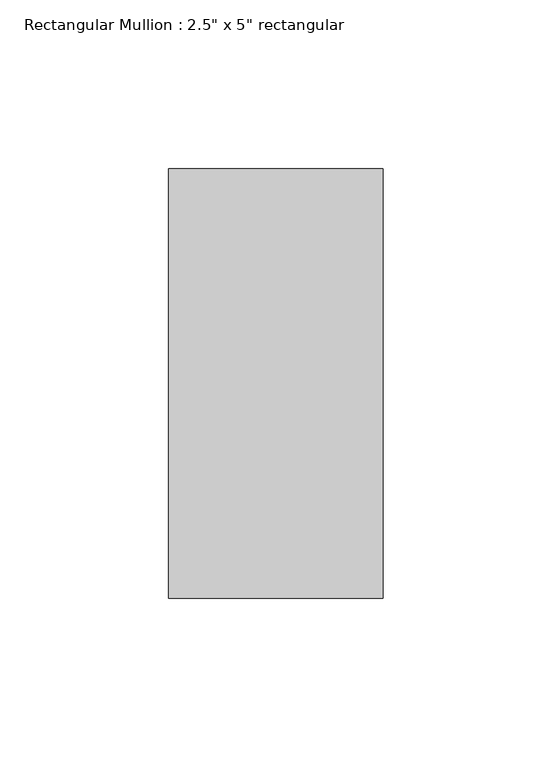
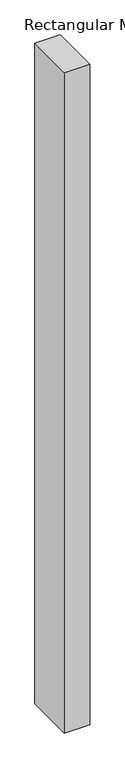
"""IFC4 building model written with IfcOpenShell, lengths in millimetres: member geometry."""

from ifc_helpers import new_model, si_unit, frame, origin, place, context, project, spatial, polyline, outline, extrude, source, transform, mapped, element, save


def member_293a584d(model_context):
    return source(origin(), model_context, "Body", "SweptSolid", [
        extrude(outline(polyline([(0.0, 63.5), (0.0, -63.5), (-63.5, -63.5), (-63.5, 63.5), (0.0, 63.5)])), frame((0.0, 0.0, -1741.7653418), z_axis=(0.0, 0.0, 1.0), x_axis=(1.0, 0.0, 0.0)), (0.0, 0.0, 1.0), 1741.7653418),
    ])


if __name__ == "__main__":
    model = new_model("IFC4")
    model_context = context("Model", 3, world=origin())
    ifc_project = project(units=[si_unit("LENGTHUNIT", "METRE", prefix="MILLI")], contexts=[model_context])
    site = spatial("IfcSite", under=ifc_project)
    building = spatial("IfcBuilding", under=site)
    placement = place(None, origin())
    member_shape = member_293a584d(model_context)
    element("IfcMember", 1, ObjectType="Rectangular Mullion : 2.5\" x 5\" rectangular", at=placement, inside=building, context=model_context, shape_type="MappedRepresentation", body=[
        mapped(member_shape, transform((0.0, 0.0, 0.0), x_axis=(1.0, 0.0, 0.0), y_axis=(0.0, 1.0, 0.0), z_axis=(0.0, 0.0, 1.0))),
    ])
    save(model, "model.ifc")

# Revit data of these elements
# Type "Rectangular Mullion : 2.5\" x 5\" rectangular"
#   built-in parameter 1007304 = 0.416667 (stored number, unit not read)
#   built-in parameter 1007301 = 0.104167 (stored number, unit not read)
#   built-in parameter 1007300 = 0.104167 (stored number, unit not read)
# Element 1 (IfcMember, "Rectangular Mullion : 2.5\" x 5\" rectangular")
#   Materials on its faces: "Aluminum"
# Materials
#   "Aluminum": class "Metal", colour RGB 247 247 247, transparency 0, Description = "Aluminum 6061", Cost = 0
